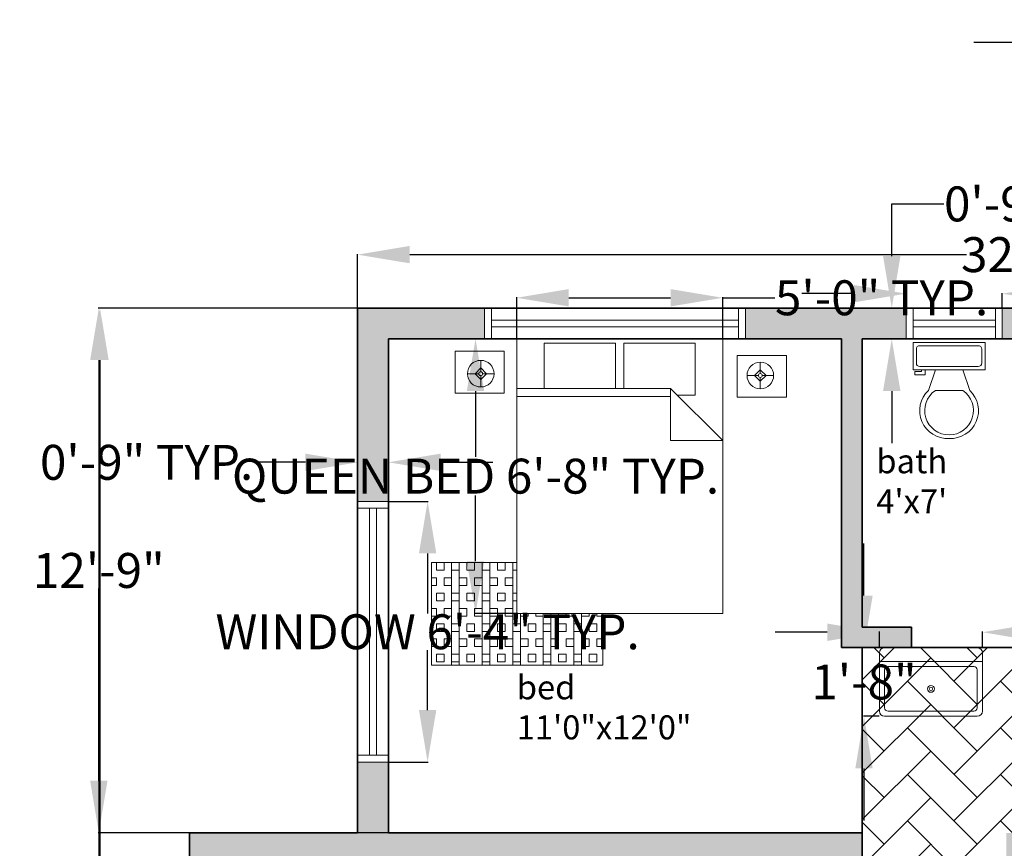
# Model space of a CAD drawing. Units: inches. Extents: x 1031 to 1706, y 87 to 654.
# Tile 2 of 4: x 1031 to 1318, y 413 to 654. Entities that reach past the tile are written whole.
import ezdxf

# ---------------------------------------------------------------- set-up
doc = ezdxf.new("R2010")
doc.units = ezdxf.units.IN
doc.header["$MEASUREMENT"] = 0
for name, color, linetype, lineweight in [('A-ANNO-DIMS', 2, 'Continuous', 18), ('A-AREA-IDEN', 7, 'Continuous', 25), ('A-FLOR-FIXT', 114, 'Continuous', 18), ('A-FLOR-PATT', 152, 'Continuous', 13), ('A-FURN', 215, 'Continuous', 18), ('A-GLAZ', 4, 'Continuous', 18), ('A-WALL', 7, 'Continuous', 35), ('A-WALL-PATT', 18, 'Continuous', 13)]:
    doc.layers.add(name, color=color, linetype=linetype, lineweight=lineweight)
doc.styles.get("Standard").update_dxf_attribs({"font": 'arial.ttf'})
doc.dimstyles.get("Standard").update_dxf_attribs({"dimtxt": 10.18, "dimasz": 15.18, "dimexe": 0.18, "dimexo": 0.0625, "dimgap": 0.09, "dimtad": 0, "dimtih": 1, "dimtoh": 1, "dimdec": 0, "dimzin": 0, "dimdsep": 46, "dimlunit": 3, "dimtxsty": 'Standard', "dimcen": 0.09, "dimadec": 0, "dimazin": 0, "dimtfac": 1, "dimtdec": 0, "dimtofl": 0, "dimtmove": 0, "dimatfit": 3, "dimfxl": 1, "dimtolj": 1, "dimtzin": 0, "dimarcsym": 0})

# ---------------------------------------------------------------- blocks, each defined once
blk = doc.blocks.new('Sink-single - 30 in top')
blk.add_line((-15, -3.999996), (15, -3.999996))
for points in [[(-13.5, 0), (13.5, 0)], [(-15, -18.499996), (-15, -1.5)], [(15, -1.5), (15, -18.499996)], [(-12.5, -5.499996), (12.5, -5.499996)], [(-13.5, -17.499996), (-13.5, -6.499996)], [(13.5, -6.499996), (13.5, -17.499996)], [(13.5, -19.999996), (-13.5, -19.999996)], [(12.5, -18.499996), (-12.5, -18.499996)]]:
    blk.add_lwpolyline(points)
for radius in [1, 0.5]:
    blk.add_circle((0, -11.999996), radius)
for centre, radius, start, end in [((-13.5, -1.5), 1.5, 90, 180), ((13.5, -1.5), 1.5, 0, 90), ((-12.5, -6.499996), 1, 90, 180), ((12.5, -6.499996), 1, 0, 90), ((-13.5, -18.499996), 1.5, 180, 270), ((-12.5, -17.499996), 1, 180, 270), ((12.5, -17.499996), 1, 270, 0), ((13.5, -18.499996), 1.5, 270, 0)]:
    blk.add_arc(centre, radius, start, end)
blk = doc.blocks.new('Bed - Queen')
for p, q in [((0, -80.00003), (0, 0)), ((0, 0), (59.99999, 0)), ((59.99999, 0), (59.99999, -80.00003)), ((7.99999, -1.2), (28.79998, -1.2)), ((7.99999, -14.4), (7.99999, -1.2)), ((28.79998, -1.2), (28.79998, -14.4)), ((31.19999, -1.2), (51.99999, -1.2)), ((31.19999, -14.4), (31.19999, -1.2)), ((51.99999, -1.2), (51.99999, -16.4)), ((0, -14.4), (44.8, -14.4)), ((44.8, -16.8), (0, -16.8)), ((59.99999, -29.6), (44.8, -14.4)), ((44.8, -14.4), (44.8, -29.6)), ((51.99999, -16.4), (46.79936, -16.4)), ((44.8, -29.6), (59.99999, -29.6)), ((59.99999, -80.00003), (0, -80.00003))]:
    blk.add_line(p, q)
blk = doc.blocks.new('Lamp - Table')
for p, q in [((0, 7), (0, 1)), ((-1, 0), (-7, 0)), ((0, 3), (-3, 0)), ((-3, 0), (0, -3)), ((3, 0), (0, 3)), ((0, -3), (3, 0)), ((1, 0), (7, 0)), ((0, -1), (0, -7))]:
    blk.add_line(p, q)
for radius in [7, 1]:
    blk.add_circle((0, 0), radius)
blk = doc.blocks.new('*U11')
for p, q in [((9.5, -6), (9.5, -2)), ((-10, -8.5), (-8, -8.5)), ((-10, -9.5), (-10, -8.5)), ((-8, -8.5), (-8, -8)), ((-7, -8), (-7, -9.5)), ((-4, -8), (-6, -14)), ((4, -8), (6, -14)), ((-7, -9.5), (-10, -9.5)), ((4, -14), (-4, -14))]:
    blk.add_line(p, q)
blk.add_lwpolyline([(10.5, -8), (10.5, 0), (-10.5, 0), (-10.5, -8)], close=True)
for points in [[(-9.5, -2), (-9.5, -6)], [(8.5, -1), (-8.5, -1)], [(-8.5, -7), (8.5, -7)]]:
    blk.add_lwpolyline(points)
for centre, radius, start, end in [((-8.625, -1.875), 0.8839, 81.8699, 188.1301), ((8.625, -1.875), 0.8839, 351.8699, 98.1301), ((-8.625, -6.125), 0.8839, 171.869898, 278.1301), ((8.625, -6.125), 0.8839, 261.8699, 8.1301), ((-0.4772, -19.9188), 8.0953, 133.01722, 273.38), ((0.0374, -19.8731), 7.127, 124.50543, 269.7), ((-0.0373, -19.8731), 7.127, 270.3, 55.4946), ((0.4773, -19.9188), 8.0953, 266.62, 46.9828)]:
    blk.add_arc(centre, radius, start, end)
blk = doc.blocks.new('*D12')
at = {"layer": 'A-ANNO-DIMS', "color": 0, "lineweight": -2, "transparency": 16777216}
for p, q in [((1129.6, 570.46), (1129.6, 586.16)), ((1144.78, 585.98), (1307.03, 585.98)), ((1504.42, 585.98), (1342.17, 585.98)), ((1519.6, 570.46), (1519.6, 586.16))]:
    blk.add_line(p, q, dxfattribs=at)
at = {"layer": 'A-ANNO-DIMS', "color": 0, "transparency": 16777216}
for points in [[(1144.78, 588.51), (1144.78, 583.45), (1129.6, 585.98)], [(1504.42, 588.51), (1504.42, 583.45), (1519.6, 585.98)]]:
    blk.add_solid(points, dxfattribs=at)
at = {"layer": 'Defpoints', "color": 0, "transparency": 16777216}
for p in [(1519.6, 585.98), (1129.6, 570.4), (1519.6, 570.4)]:
    blk.add_point(p, dxfattribs=at)
at = {"layer": 'A-ANNO-DIMS', "color": 0, "transparency": 16777216, "insert": (1324.6, 585.98), "char_height": 10.18, "attachment_point": 5}
blk.add_mtext('\\A1;32\'-6"', dxfattribs=at)
blk = doc.blocks.new('*D13')
at = {"layer": 'A-ANNO-DIMS', "color": 0, "lineweight": -2, "transparency": 16777216}
for p, q in [((1129.54, 570.4), (1054.37, 570.4)), ((1054.55, 555.22), (1054.55, 383.69)), ((1054.55, 201.58), (1054.55, 373.11)), ((1129.54, 186.4), (1054.37, 186.4))]:
    blk.add_line(p, q, dxfattribs=at)
at = {"layer": 'A-ANNO-DIMS', "color": 0, "transparency": 16777216}
for points in [[(1052.02, 555.22), (1057.08, 555.22), (1054.55, 570.4)], [(1052.02, 201.58), (1057.08, 201.58), (1054.55, 186.4)]]:
    blk.add_solid(points, dxfattribs=at)
at = {"layer": 'Defpoints', "color": 0, "transparency": 16777216}
for p in [(1129.6, 570.4), (1054.55, 186.4), (1129.6, 186.4)]:
    blk.add_point(p, dxfattribs=at)
at = {"layer": 'A-ANNO-DIMS', "color": 0, "transparency": 16777216, "insert": (1054.55, 378.4), "char_height": 10.18, "attachment_point": 5}
blk.add_mtext("\\A1;32'", dxfattribs=at)
blk = doc.blocks.new('WIN-72IN')
for p, q in [((0, 0), (0, 9)), ((2, 0), (2, 9)), ((74, 0), (74, 9)), ((76, 0), (76, 9)), ((2, 5.5), (74, 5.5)), ((2, 3.5), (74, 3.5))]:
    blk.add_line(p, q)
blk = doc.blocks.new('WIN-24IN')
for p, q in [((0, 0), (0, 9)), ((2, 0), (2, 9)), ((26, 0), (26, 9)), ((28, 0), (28, 9)), ((2, 5.5), (26, 5.5)), ((2, 3.5), (26, 3.5))]:
    blk.add_line(p, q)
blk = doc.blocks.new('NIGHTSTAND-RECT')
blk.add_lwpolyline([(0, 12.21), (14.36, 12.21), (14.36, 0), (0, 0)], close=True)
blk = doc.blocks.new('*D18')
at = {"layer": 'A-ANNO-DIMS', "color": 0, "lineweight": -2, "transparency": 16777216}
for p, q in [((1138.66, 514.03), (1150.18, 514.03)), ((1150, 498.85), (1150, 481.38)), ((1150, 453.21), (1150, 470.67)), ((1138.66, 438.03), (1150.18, 438.03))]:
    blk.add_line(p, q, dxfattribs=at)
at = {"layer": 'A-ANNO-DIMS', "color": 0, "transparency": 16777216}
for points in [[(1147.47, 498.85), (1152.53, 498.85), (1150, 514.03)], [(1147.47, 453.21), (1152.53, 453.21), (1150, 438.03)]]:
    blk.add_solid(points, dxfattribs=at)
at = {"layer": 'Defpoints', "color": 0, "transparency": 16777216}
for p in [(1138.6, 514.03), (1150, 514.03), (1138.6, 438.03)]:
    blk.add_point(p, dxfattribs=at)
at = {"layer": 'A-ANNO-DIMS', "color": 0, "transparency": 16777216, "insert": (1150, 476.03), "char_height": 10.18, "attachment_point": 5}
blk.add_mtext('\\A1;WINDOW 6\'-4" TYP.', dxfattribs=at)
blk = doc.blocks.new('*D19')
at = {"layer": 'A-ANNO-DIMS', "color": 0, "lineweight": -2, "transparency": 16777216}
for p, q in [((1114.42, 525.43), (1099.24, 525.43)), ((1129.6, 514.09), (1129.6, 525.61)), ((1138.6, 514.09), (1138.6, 525.61)), ((1153.78, 525.43), (1168.96, 525.43))]:
    blk.add_line(p, q, dxfattribs=at)
at = {"layer": 'A-ANNO-DIMS', "color": 0, "transparency": 16777216}
for points in [[(1114.42, 527.96), (1114.42, 522.9), (1129.6, 525.43)], [(1153.78, 527.96), (1153.78, 522.9), (1138.6, 525.43)]]:
    blk.add_solid(points, dxfattribs=at)
at = {"layer": 'Defpoints', "color": 0, "transparency": 16777216}
for p in [(1129.6, 525.43), (1129.6, 514.03), (1138.6, 514.03)]:
    blk.add_point(p, dxfattribs=at)
at = {"layer": 'A-ANNO-DIMS', "color": 0, "transparency": 16777216, "insert": (1068.13, 525.43), "char_height": 10.18, "attachment_point": 5}
blk.add_mtext('\\A1;0\'-9" TYP.', dxfattribs=at)
blk = doc.blocks.new('*D20')
at = {"layer": 'A-ANNO-DIMS', "color": 0, "lineweight": -2, "transparency": 16777216}
for p, q in [((1274.24, 574.6), (1259.06, 574.6)), ((1289.42, 570.46), (1289.42, 574.78)), ((1317.42, 570.46), (1317.42, 574.78)), ((1332.6, 574.6), (1347.78, 574.6))]:
    blk.add_line(p, q, dxfattribs=at)
at = {"layer": 'A-ANNO-DIMS', "color": 0, "transparency": 16777216}
for points in [[(1274.24, 577.13), (1274.24, 572.07), (1289.42, 574.6)], [(1332.6, 577.13), (1332.6, 572.07), (1317.42, 574.6)]]:
    blk.add_solid(points, dxfattribs=at)
at = {"layer": 'Defpoints', "color": 0, "transparency": 16777216}
for p in [(1317.42, 574.6), (1289.42, 570.4), (1317.42, 570.4)]:
    blk.add_point(p, dxfattribs=at)
at = {"layer": 'A-ANNO-DIMS', "color": 0, "transparency": 16777216, "insert": (1412.28, 574.6), "char_height": 10.18, "attachment_point": 5}
blk.add_mtext('\\A1;WINDOW 2\'-4" TYP.', dxfattribs=at)
blk = doc.blocks.new('*D21')
at = {"layer": 'A-ANNO-DIMS', "color": 0, "lineweight": -2, "transparency": 16777216}
for p, q in [((1285.22, 585.58), (1285.22, 600.76)), ((1285.22, 600.76), (1300.4, 600.76)), ((1289.36, 570.4), (1285.04, 570.4)), ((1289.36, 561.4), (1285.04, 561.4)), ((1285.22, 546.22), (1285.22, 531.04))]:
    blk.add_line(p, q, dxfattribs=at)
at = {"layer": 'A-ANNO-DIMS', "color": 0, "transparency": 16777216}
for points in [[(1282.69, 585.58), (1287.75, 585.58), (1285.22, 570.4)], [(1282.69, 546.22), (1287.75, 546.22), (1285.22, 561.4)]]:
    blk.add_solid(points, dxfattribs=at)
at = {"layer": 'Defpoints', "color": 0, "transparency": 16777216}
for p in [(1285.22, 570.4), (1289.42, 570.4), (1289.42, 561.4)]:
    blk.add_point(p, dxfattribs=at)
at = {"layer": 'A-ANNO-DIMS', "color": 0, "transparency": 16777216, "insert": (1331.51, 600.76), "char_height": 10.18, "attachment_point": 5}
blk.add_mtext('\\A1;0\'-9" TYP.', dxfattribs=at)
blk = doc.blocks.new('*D22')
at = {"layer": 'A-ANNO-DIMS', "color": 0, "lineweight": -2, "transparency": 16777216}
for p, q in [((1175.9, 561.4), (1163.78, 561.4)), ((1163.96, 546.22), (1163.96, 527.06)), ((1163.96, 496.58), (1163.96, 515.73)), ((1175.9, 481.4), (1163.78, 481.4))]:
    blk.add_line(p, q, dxfattribs=at)
at = {"layer": 'A-ANNO-DIMS', "color": 0, "transparency": 16777216}
for points in [[(1161.43, 546.22), (1166.49, 546.22), (1163.96, 561.4)], [(1161.43, 496.58), (1166.49, 496.58), (1163.96, 481.4)]]:
    blk.add_solid(points, dxfattribs=at)
at = {"layer": 'Defpoints', "color": 0, "transparency": 16777216}
for p in [(1163.96, 561.4), (1175.96, 561.4), (1175.96, 481.4)]:
    blk.add_point(p, dxfattribs=at)
at = {"layer": 'A-ANNO-DIMS', "color": 0, "transparency": 16777216, "insert": (1163.96, 521.4), "char_height": 10.18, "attachment_point": 5}
blk.add_mtext('\\A1;QUEEN BED 6\'-8" TYP.', dxfattribs=at)
blk = doc.blocks.new('*D23')
at = {"layer": 'A-ANNO-DIMS', "color": 0, "lineweight": -2, "transparency": 16777216}
for p, q in [((1175.96, 561.46), (1175.96, 573.58)), ((1191.14, 573.4), (1220.78, 573.4)), ((1235.96, 561.46), (1235.96, 573.58)), ((1235.96, 573.4), (1251.14, 573.4))]:
    blk.add_line(p, q, dxfattribs=at)
at = {"layer": 'A-ANNO-DIMS', "color": 0, "transparency": 16777216}
for points in [[(1191.14, 575.93), (1191.14, 570.87), (1175.96, 573.4)], [(1220.78, 575.93), (1220.78, 570.87), (1235.96, 573.4)]]:
    blk.add_solid(points, dxfattribs=at)
at = {"layer": 'Defpoints', "color": 0, "transparency": 16777216}
for p in [(1235.96, 573.4), (1175.96, 561.4), (1235.96, 561.4)]:
    blk.add_point(p, dxfattribs=at)
at = {"layer": 'A-ANNO-DIMS', "color": 0, "transparency": 16777216, "insert": (1282.26, 573.4), "char_height": 10.18, "attachment_point": 5}
blk.add_mtext('\\A1;5\'-0" TYP.', dxfattribs=at)
blk = doc.blocks.new('*D32')
at = {"layer": 'A-ANNO-DIMS', "color": 0, "lineweight": -2, "transparency": 16777216}
for p, q in [((1266.45, 475.89), (1251.27, 475.89)), ((1281.63, 471.45), (1281.63, 476.07)), ((1311.63, 471.45), (1311.63, 476.07)), ((1326.81, 475.89), (1341.99, 475.89))]:
    blk.add_line(p, q, dxfattribs=at)
at = {"layer": 'A-ANNO-DIMS', "color": 0, "transparency": 16777216}
for points in [[(1266.45, 478.42), (1266.45, 473.36), (1281.63, 475.89)], [(1326.81, 478.42), (1326.81, 473.36), (1311.63, 475.89)]]:
    blk.add_solid(points, dxfattribs=at)
at = {"layer": 'Defpoints', "color": 0, "transparency": 16777216}
for p in [(1311.63, 475.89), (1281.63, 471.39), (1311.63, 471.39)]:
    blk.add_point(p, dxfattribs=at)
at = {"layer": 'A-ANNO-DIMS', "color": 0, "transparency": 16777216, "insert": (1378.7, 475.89), "char_height": 10.18, "attachment_point": 5}
blk.add_mtext('\\A1;BASIN 2\'-6"', dxfattribs=at)
blk = doc.blocks.new('*D33')
at = {"layer": 'A-ANNO-DIMS', "color": 0, "lineweight": -2, "transparency": 16777216}
for p, q in [((1277.13, 486.57), (1277.13, 501.75)), ((1281.56, 471.39), (1276.95, 471.39)), ((1281.56, 451.39), (1276.95, 451.39)), ((1277.13, 436.21), (1277.13, 421.03))]:
    blk.add_line(p, q, dxfattribs=at)
at = {"layer": 'A-ANNO-DIMS', "color": 0, "transparency": 16777216}
for points in [[(1274.6, 486.57), (1279.66, 486.57), (1277.13, 471.39)], [(1274.6, 436.21), (1279.66, 436.21), (1277.13, 451.39)]]:
    blk.add_solid(points, dxfattribs=at)
at = {"layer": 'Defpoints', "color": 0, "transparency": 16777216}
for p in [(1277.13, 471.39), (1281.63, 471.39), (1281.63, 451.39)]:
    blk.add_point(p, dxfattribs=at)
at = {"layer": 'A-ANNO-DIMS', "color": 0, "transparency": 16777216, "insert": (1277.13, 461.39), "char_height": 10.18, "attachment_point": 5}
blk.add_mtext('\\A1;1\'-8"', dxfattribs=at)
blk = doc.blocks.new('*D41')
at = {"layer": 'A-ANNO-DIMS', "color": 0, "lineweight": -2, "transparency": 16777216}
for p, q in [((1129.54, 570.4), (1054.03, 570.4)), ((1054.21, 555.22), (1054.21, 354.79)), ((1054.21, 143.78), (1054.21, 344.21)), ((1324.54, 128.6), (1054.03, 128.6))]:
    blk.add_line(p, q, dxfattribs=at)
at = {"layer": 'A-ANNO-DIMS', "color": 0, "transparency": 16777216}
for points in [[(1051.68, 555.22), (1056.74, 555.22), (1054.21, 570.4)], [(1051.68, 143.78), (1056.74, 143.78), (1054.21, 128.6)]]:
    blk.add_solid(points, dxfattribs=at)
at = {"layer": 'Defpoints', "color": 0, "transparency": 16777216}
for p in [(1054.21, 570.4), (1129.6, 570.4), (1324.6, 128.6)]:
    blk.add_point(p, dxfattribs=at)
at = {"layer": 'A-ANNO-DIMS', "color": 0, "transparency": 16777216, "insert": (1054.21, 349.5), "char_height": 10.18, "attachment_point": 5}
blk.add_mtext('\\A1;36\'-10"', dxfattribs=at)
blk = doc.blocks.new('*D42')
at = {"layer": 'A-ANNO-DIMS', "color": 0, "lineweight": -2, "transparency": 16777216}
for p, q in [((1289.36, 570.4), (1054.03, 570.4)), ((1054.21, 555.22), (1054.21, 499.19)), ((1054.21, 432.58), (1054.21, 488.61)), ((1276.54, 417.4), (1054.03, 417.4))]:
    blk.add_line(p, q, dxfattribs=at)
at = {"layer": 'A-ANNO-DIMS', "color": 0, "transparency": 16777216}
for points in [[(1051.68, 555.22), (1056.74, 555.22), (1054.21, 570.4)], [(1051.68, 432.58), (1056.74, 432.58), (1054.21, 417.4)]]:
    blk.add_solid(points, dxfattribs=at)
at = {"layer": 'Defpoints', "color": 0, "transparency": 16777216}
for p in [(1054.21, 570.4), (1289.42, 570.4), (1276.6, 417.4)]:
    blk.add_point(p, dxfattribs=at)
at = {"layer": 'A-ANNO-DIMS', "color": 0, "transparency": 16777216, "insert": (1054.21, 493.9), "char_height": 10.18, "attachment_point": 5}
blk.add_mtext('\\A1;12\'-9"', dxfattribs=at)
blk = doc.blocks.new('*D44')
at = {"layer": 'A-ANNO-DIMS', "color": 0, "lineweight": -2, "transparency": 16777216}
for p, q in [((1324.29, 647.8), (1309.11, 647.8)), ((1339.47, 561.46), (1339.47, 647.98)), ((1360.47, 561.46), (1360.47, 647.98)), ((1375.65, 647.8), (1390.83, 647.8))]:
    blk.add_line(p, q, dxfattribs=at)
at = {"layer": 'A-ANNO-DIMS', "color": 0, "transparency": 16777216}
for points in [[(1324.29, 650.33), (1324.29, 645.27), (1339.47, 647.8)], [(1375.65, 650.33), (1375.65, 645.27), (1360.47, 647.8)]]:
    blk.add_solid(points, dxfattribs=at)
at = {"layer": 'Defpoints', "color": 0, "transparency": 16777216}
for p in [(1360.47, 647.8), (1339.47, 561.4), (1360.47, 561.4)]:
    blk.add_point(p, dxfattribs=at)
at = {"layer": 'A-ANNO-DIMS', "color": 0, "transparency": 16777216, "insert": (1403.97, 647.8), "char_height": 10.18, "attachment_point": 5}
blk.add_mtext('\\A1;1\'-9"', dxfattribs=at)

msp = doc.modelspace()

# ---------------------------------------------------------------- hatches: boundary and pattern name
at = {"layer": 'A-FLOR-PATT'}
h = msp.add_hatch(dxfattribs=at)
h.set_pattern_fill('AR-HBONE', color=256, scale=2.4)
h.paths.add_polyline_path([(1372.6, 507.4), (1330.6, 507.4), (1330.6, 471.4), (1276.6, 471.4), (1276.6, 408.4), (1276.6, 336.4), (1318.6, 336.4), (1318.6, 417.4), (1372.6, 417.4)])
h = msp.add_hatch(dxfattribs=at)
h.set_pattern_fill('BOX', color=256, scale=8.9)
h.paths.add_polyline_path([(1201.04, 481.4), (1175.96, 481.4), (1175.96, 496.22), (1151.17, 496.22), (1151.17, 466.33), (1201.04, 466.33)])
at = {"layer": 'A-WALL-PATT'}
h = msp.add_hatch(color=256, dxfattribs=at)
h.dxf.hatch_style = 1
h.paths.add_polyline_path([(1324.6, 336.4), (1318.6, 336.4), (1318.6, 327.4), (1318.6, 195.4), (1256.53, 195.4), (1256.53, 186.4), (1316.43, 186.4), (1316.43, 128.6), (1324.6, 128.6), (1324.6, 142.78), (1421.89, 142.78), (1421.89, 143.49), (1324.6, 143.49), (1324.6, 157.67), (1324.6, 171.8), (1421.89, 171.8), (1421.89, 172.21), (1324.6, 172.21), (1324.6, 186.4)])
h.paths.add_polyline_path([(1378.07, 258.4), (1358.04, 258.4), (1358.04, 249.4), (1378.07, 249.4)], flags=17)
h.paths.add_polyline_path([(1519.6, 299.69), (1510.6, 299.69), (1510.6, 258.4), (1454.07, 258.4), (1454.07, 249.4), (1519.6, 249.4)])
h.paths.add_polyline_path([(1519.6, 456.87), (1510.6, 456.87), (1510.6, 417.4), (1372.6, 417.4), (1318.6, 417.4), (1318.6, 408.4), (1510.6, 408.4), (1510.6, 375.69), (1519.6, 375.69)])
h.paths.add_polyline_path([(1276.6, 372.4), (1270.65, 372.4), (1270.65, 336.4), (1138.6, 336.4), (1092.08, 336.4), (1092.08, 346.4), (1080.61, 346.4), (1080.61, 327.4), (1129.6, 327.4), (1129.6, 290.93), (1138.6, 290.93), (1138.6, 291.84), (1138.6, 327.4), (1244.94, 327.4), (1276.6, 327.4)])
h.paths.add_polyline_path([(1276.6, 417.4), (1138.6, 417.4), (1138.6, 438.03), (1129.6, 438.03), (1129.6, 417.4), (1080.61, 417.4), (1080.61, 398.4), (1092.08, 398.4), (1092.08, 408.4), (1138.6, 408.4), (1276.6, 408.4)])
h.paths.add_polyline_path([(1180.53, 195.4), (1138.6, 195.4), (1138.6, 214.93), (1129.6, 214.93), (1129.6, 186.4), (1180.53, 186.4)])
h.paths.add_polyline_path([(1519.6, 570.4), (1489.02, 570.4), (1489.02, 561.4), (1510.6, 561.4), (1510.6, 532.87), (1519.6, 532.87)])
h.paths.add_polyline_path([(1413.02, 570.4), (1365.47, 570.4), (1365.47, 561.4), (1372.6, 561.4), (1372.6, 507.4), (1372.6, 417.4), (1378.6, 417.4), (1378.6, 561.4), (1413.02, 561.4)])
h.paths.add_polyline_path([(1289.42, 570.4), (1242.6, 570.4), (1242.6, 561.4), (1270.6, 561.4), (1270.6, 471.4), (1291.02, 471.4), (1291.02, 477.4), (1276.6, 477.4), (1276.6, 561.4), (1289.42, 561.4)])
h.paths.add_polyline_path([(1337.47, 570.4), (1317.42, 570.4), (1317.42, 561.4), (1324.6, 561.4), (1324.6, 471.4), (1330.6, 471.4), (1330.6, 507.4), (1338.54, 507.4), (1338.54, 513.4), (1330.6, 513.4), (1330.6, 561.4), (1337.47, 561.4)])
h.paths.add_polyline_path([(1138.6, 561.4), (1166.6, 561.4), (1166.6, 570.4), (1129.6, 570.4), (1129.6, 514.03), (1138.6, 514.03)])

# ---------------------------------------------------------------- linework, layer by layer
at = {"layer": 'A-FURN'}
for p, q in [((1175.96, 496.22), (1151.17, 496.22)), ((1151.17, 496.22), (1151.17, 466.33)), ((1175.96, 496.22), (1175.96, 496.22)), ((1201.04, 466.33), (1201.04, 481.4)), ((1151.17, 466.33), (1201.04, 466.33))]:
    msp.add_line(p, q, dxfattribs=at)
at = {"layer": 'A-WALL'}
for p, q in [((1129.6, 570.4), (1519.6, 570.4)), ((1129.6, 417.4), (1129.6, 570.4)), ((1138.6, 561.4), (1270.6, 561.4)), ((1138.6, 417.4), (1138.6, 561.4)), ((1270.6, 471.4), (1270.6, 561.4)), ((1276.6, 477.4), (1276.6, 561.4)), ((1276.6, 561.4), (1324.6, 561.4)), ((1276.6, 477.4), (1291.02, 477.4)), ((1291.02, 477.4), (1291.02, 471.4)), ((1270.6, 471.4), (1330.6, 471.4)), ((1276.6, 408.4), (1276.6, 471.4)), ((1129.6, 417.4), (1080.61, 417.4)), ((1080.61, 417.4), (1080.61, 327.4)), ((1138.6, 417.4), (1276.6, 417.4))]:
    msp.add_line(p, q, dxfattribs=at)

# ---------------------------------------------------------------- block references
at = {"layer": 'A-FLOR-FIXT'}
for name, p in [('*U11', (1301.92, 560.4)), ('Sink-single - 30 in top', (1296.63, 471.39))]:
    msp.add_blockref(name, p, dxfattribs=at)
at = {"layer": 'A-FURN'}
for name, p in [('Bed - Queen', (1175.96, 561.4)), ('NIGHTSTAND-RECT', (1157.99, 545.63)), ('NIGHTSTAND-RECT', (1240.18, 544.41))]:
    msp.add_blockref(name, p, dxfattribs=at)
at = {"layer": 'A-FURN', "xscale": 0.5540798285396209, "yscale": 0.5540798285396209, "zscale": 0.5540798285396209}
for p in [(1165.47, 551.27), (1246.93, 550.75)]:
    msp.add_blockref('Lamp - Table', p, dxfattribs=at)
at = {"layer": 'A-GLAZ'}
for name, p in [('WIN-72IN', (1166.6, 561.4)), ('WIN-24IN', (1289.42, 561.4))]:
    msp.add_blockref(name, p, dxfattribs=at)
at = {"layer": 'A-GLAZ', "rotation": 90.00000000000018}
msp.add_blockref('WIN-72IN', (1138.6, 438.03), dxfattribs=at)

# ---------------------------------------------------------------- texts
at = {"layer": 'A-AREA-IDEN', "char_height": 7, "attachment_point": 1}
for s, insert in [("bath\\P4'x7'", (1280.71, 529.24)), ('bed\\P11\'0"x12\'0"', (1175.96, 463.33))]:
    msp.add_mtext_dynamic_manual_height_columns(s, width=113.8004, gutter_width=1, heights=[0], dxfattribs=dict(at, insert=insert))

# ---------------------------------------------------------------- dimensions: what is measured, and where the dimension line sits
at = {"layer": 'A-ANNO-DIMS'}
for base, p1, p2, override, picture, middle in [((1360.47, 647.8), (1339.47, 561.4), (1360.47, 561.4), {"dimdec": 1, "dimlfac": 1, "dimrnd": 0, "dimzin": 1, "dimdsep": 46, "dimlunit": 4, "dimfrac": 2}, '*D44', (1403.97, 647.8)), ((1519.6, 585.98), (1129.6, 570.4), (1519.6, 570.4), {"dimclrd": 0, "dimclre": 0, "dimclrt": 0}, '*D12', (1324.6, 585.98))]:
    dim = msp.add_linear_dim(base=base, p1=p1, p2=p2, dimstyle='Standard', override=override, dxfattribs=at)
    dim.commit()
    dim.dimension.update_dxf_attribs({"geometry": picture, "text_midpoint": middle})
for base, p1, p2, angle, text, picture, middle in [((1285.22, 570.4), (1289.42, 561.4), (1289.42, 570.4), 90, '<> TYP.', '*D21', (1331.51, 600.76)), ((1163.96, 561.4), (1175.96, 481.4), (1175.96, 561.4), 90, 'QUEEN BED <> TYP.', '*D22', (1163.96, 521.4)), ((1129.6, 525.43), (1138.6, 514.03), (1129.6, 514.03), 180, '<> TYP.', '*D19', (1068.13, 525.43)), ((1150, 514.03), (1138.6, 438.03), (1138.6, 514.03), 90, 'WINDOW <> TYP.', '*D18', (1150, 476.03))]:
    dim = msp.add_linear_dim(base=base, p1=p1, p2=p2, angle=angle, text=text, dimstyle='Standard', override={"dimdec": 1, "dimlfac": 1, "dimrnd": 0, "dimzin": 1, "dimdsep": 46, "dimlunit": 4, "dimfrac": 2}, dxfattribs=at)
    dim.commit()
    dim.dimension.update_dxf_attribs({"geometry": picture, "text_midpoint": middle})
for base, p1, p2, text, picture, middle in [((1317.42, 574.6), (1289.42, 570.4), (1317.42, 570.4), 'WINDOW <> TYP.', '*D20', (1412.28, 574.6)), ((1235.96, 573.4), (1175.96, 561.4), (1235.96, 561.4), '<> TYP.', '*D23', (1282.26, 573.4)), ((1311.63, 475.89), (1281.63, 471.39), (1311.63, 471.39), 'BASIN <>', '*D32', (1378.7, 475.89))]:
    dim = msp.add_linear_dim(base=base, p1=p1, p2=p2, text=text, dimstyle='Standard', override={"dimdec": 1, "dimlfac": 1, "dimrnd": 0, "dimzin": 1, "dimdsep": 46, "dimlunit": 4, "dimfrac": 2}, dxfattribs=at)
    dim.commit()
    dim.dimension.update_dxf_attribs({"geometry": picture, "text_midpoint": middle})
for base, p1, p2, override, picture, middle in [((1054.21, 570.4), (1324.6, 128.6), (1129.6, 570.4), {"dimdec": 1, "dimlfac": 1, "dimrnd": 0, "dimzin": 1, "dimdsep": 46, "dimlunit": 4, "dimfrac": 2}, '*D41', (1054.21, 349.5)), ((1054.21, 570.4), (1276.6, 417.4), (1289.42, 570.4), {"dimdec": 1, "dimlfac": 1, "dimrnd": 0, "dimzin": 1, "dimdsep": 46, "dimlunit": 4, "dimfrac": 2}, '*D42', (1054.21, 493.9)), ((1054.55, 186.4), (1129.6, 570.4), (1129.6, 186.4), {"dimclrd": 0, "dimclre": 0, "dimclrt": 0}, '*D13', (1054.55, 378.4)), ((1277.13, 471.39), (1281.63, 451.39), (1281.63, 471.39), {"dimdec": 1, "dimlfac": 1, "dimrnd": 0, "dimzin": 1, "dimdsep": 46, "dimlunit": 4, "dimfrac": 2}, '*D33', (1277.13, 461.39))]:
    dim = msp.add_linear_dim(base=base, p1=p1, p2=p2, angle=90, dimstyle='Standard', override=override, dxfattribs=at)
    dim.commit()
    dim.dimension.update_dxf_attribs({"geometry": picture, "text_midpoint": middle})

doc.saveas('drawing.dxf')
